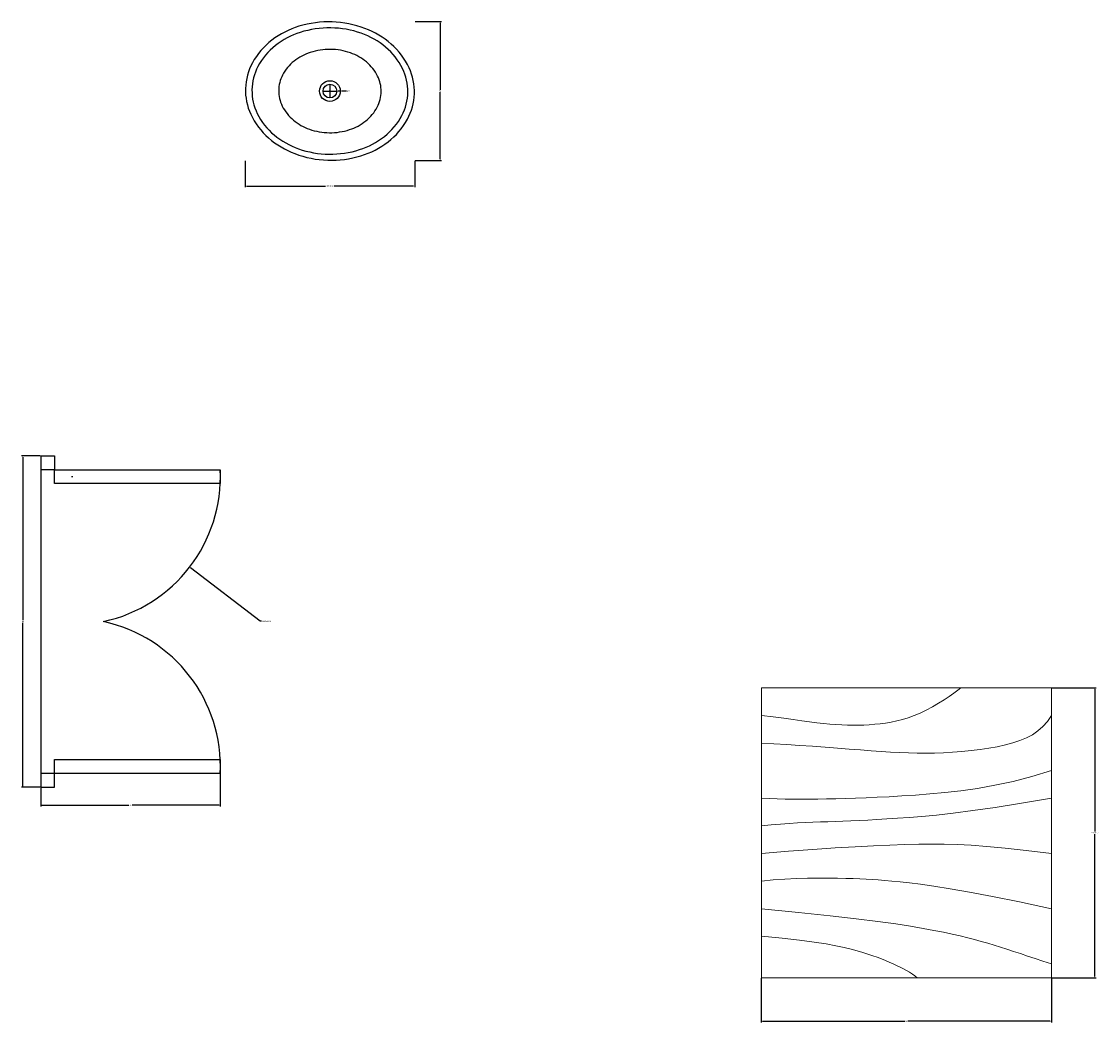
# Model space of a CAD drawing. Units: inches. Extents: x 821 to 2399, y 74 to 823.
# Tile 9 of 13: x 1922 to 2078, y 193 to 338. Entities that reach past the tile are written whole.
import ezdxf

# ---------------------------------------------------------------- set-up
doc = ezdxf.new("R2010")
doc.units = ezdxf.units.IN
doc.header["$MEASUREMENT"] = 0
doc.layers.get('0').update_dxf_attribs({"lineweight": 53})
for name, color, linetype, lineweight in [('A-ANNO-DIMS', 2, 'Continuous', 18), ('A-DOOR', 4, 'Continuous', 25), ('A-FLOR-FIXT', 8, 'Continuous', 25), ('A-FURN', 8, 'Continuous', 18)]:
    doc.layers.add(name, color=color, linetype=linetype, lineweight=lineweight)
doc.styles.get("Standard").update_dxf_attribs({"font": 'arial.ttf'})
doc.dimstyles.get("Standard").update_dxf_attribs({"dimtxt": 0.18, "dimasz": 0.18, "dimexe": 0.18, "dimexo": 0.0625, "dimgap": 0.09, "dimtad": 0, "dimtih": 1, "dimtoh": 1, "dimdec": 4, "dimzin": 0, "dimdsep": 46, "dimtxsty": 'Standard', "dimcen": 0.09, "dimadec": 0, "dimazin": 0, "dimtfac": 1, "dimtdec": 4, "dimtofl": 0, "dimtmove": 0, "dimatfit": 3, "dimfxl": 1, "dimtolj": 1, "dimtzin": 0, "dimarcsym": 0})

# ---------------------------------------------------------------- blocks, each defined once
blk = doc.blocks.new('Table - Square Woodgrain 42 x 42 in.')
blk.add_line((0, -42), (42, -42))
for points in [[(0, -4), (1.704, -4.2172), (3.2358, -4.4188), (4.615, -4.604), (5.8615, -4.7721), (6.9951, -4.9224), (8.0357, -5.0541), (9.0031, -5.1667), (9.9171, -5.2594), (10.7951, -5.3316), (11.6445, -5.3836), (12.4702, -5.4157), (13.277, -5.4283), (14.0698, -5.4217), (14.8535, -5.3964), (15.6331, -5.3526), (16.4133, -5.2908), (17.1986, -5.2103), (17.9913, -5.1062), (18.793, -4.9727), (19.6056, -4.8038), (20.4307, -4.5937), (21.2701, -4.3365), (22.1256, -4.0262), (22.9989, -3.6571), (23.888, -3.2272), (24.7756, -2.7516), (25.6408, -2.2491), (26.4624, -1.7387), (27.2195, -1.2395), (27.891, -0.7703), (28.456, -0.3501), (28.8934, 0.002)], [(0, -42), (0, 0), (42, 0), (42, -42)], [(0, -8), (1.8203, -8.1001), (3.6741, -8.2149), (5.5411, -8.3408), (7.4011, -8.4741), (9.2339, -8.6112), (11.0193, -8.7484), (12.7371, -8.8821), (14.3671, -9.0086), (15.8954, -9.1246), (17.3337, -9.2278), (18.6997, -9.3159), (20.0116, -9.387), (21.2871, -9.4389), (22.5442, -9.4696), (23.8008, -9.477), (25.0749, -9.459), (26.3791, -9.4137), (27.7049, -9.3403), (29.0383, -9.2382), (30.3655, -9.1068), (31.6728, -8.9455), (32.9461, -8.7535), (34.1717, -8.5304), (35.3358, -8.2756), (36.4268, -7.9863), (37.443, -7.6521), (38.3849, -7.2603), (39.253, -6.7986), (40.048, -6.2542), (40.7705, -5.6147), (41.421, -4.8674), (42, -4)], [(42, -12), (39.1784, -12.8621), (36.4519, -13.5654), (33.8246, -14.1294), (31.3004, -14.5731), (28.8832, -14.9161), (26.577, -15.1775), (24.3858, -15.3768), (22.3136, -15.5332), (20.3622, -15.6632), (18.5254, -15.7718), (16.7947, -15.8612), (15.1618, -15.9338), (13.6183, -15.9916), (12.1558, -16.0369), (10.7659, -16.0718), (9.4403, -16.0987), (8.1703, -16.1191), (6.9461, -16.1325), (5.7577, -16.1377), (4.595, -16.1335), (3.4479, -16.1188), (2.3064, -16.0924), (1.1604, -16.0532), (0, -16)], [(42, -16), (37.6529, -16.7365), (33.8802, -17.329), (30.6179, -17.7961), (27.8015, -18.1561), (25.3668, -18.4275), (23.2497, -18.6288), (21.3859, -18.7785), (19.7111, -18.8949), (18.1693, -18.9939), (16.7375, -19.0795), (15.401, -19.1534), (14.1449, -19.217), (12.9544, -19.2717), (11.8148, -19.3191), (10.7113, -19.3606), (9.6291, -19.3976), (8.5534, -19.4323), (7.47, -19.4689), (6.3643, -19.5122), (5.222, -19.5672), (4.0288, -19.6386), (2.7703, -19.7313), (1.4321, -19.8501), (0, -20)], [(0, -24), (3.9243, -23.6805), (7.4766, -23.4138), (10.6891, -23.1954), (13.5943, -23.0205), (16.2247, -22.8847), (18.6125, -22.7832), (20.7903, -22.7116), (22.7903, -22.6651), (24.6563, -22.642), (26.4764, -22.6507), (28.35, -22.7024), (30.3766, -22.8084), (32.6555, -22.98), (35.2861, -23.2283), (38.3678, -23.5645), (42, -24)], [(42, -32), (37.392, -31.017), (33.4585, -30.2231), (30.1291, -29.5949), (27.3334, -29.109), (25.0009, -28.742), (23.0612, -28.4707), (21.4439, -28.2716), (20.0786, -28.1215), (18.8998, -28.0002), (17.8609, -27.9014), (16.9206, -27.8219), (16.0371, -27.7588), (15.1691, -27.709), (14.2748, -27.6693), (13.3128, -27.6368), (12.2415, -27.6083), (11.0295, -27.5824), (9.6867, -27.5643), (8.233, -27.5608), (6.6884, -27.5787), (5.0728, -27.6248), (3.4062, -27.7058), (1.7086, -27.8286), (0, -28)], [(0, -32), (5.4026, -32.5358), (9.9494, -33.019), (13.7424, -33.4553), (16.8834, -33.8505), (19.4743, -34.2106), (21.6171, -34.5413), (23.4136, -34.8486), (24.9657, -35.1382), (26.3614, -35.4156), (27.6332, -35.6841), (28.7995, -35.9467), (29.8788, -36.2064), (30.8897, -36.4661), (31.8507, -36.7288), (32.7802, -36.9973), (33.6968, -37.2747), (34.6175, -37.5635), (35.5531, -37.8651), (36.5128, -38.1805), (37.506, -38.5108), (38.5421, -38.8568), (39.6302, -39.2197), (40.7797, -39.6004), (42, -40)], [(0, -36), (3.0098, -36.2857), (5.5354, -36.5643), (7.6368, -36.8359), (9.374, -37.1009), (10.807, -37.3597), (11.9957, -37.6126), (13.0002, -37.8599), (13.8804, -38.102), (14.6874, -38.3393), (15.4365, -38.5729), (16.1338, -38.8041), (16.7858, -39.0341), (17.3987, -39.264), (17.9787, -39.4952), (18.5322, -39.7288), (19.0655, -39.9662), (19.5832, -40.2081), (20.0842, -40.4544), (20.5657, -40.7046), (21.0249, -40.9581), (21.459, -41.2144), (21.8653, -41.4731), (22.2409, -41.7335), (22.5831, -41.9951)]]:
    blk.add_lwpolyline(points)
blk = doc.blocks.new('Sink - Oval top')
for p, q in [((-1, 0), (1, 0)), ((0, 1), (0, -1))]:
    blk.add_line(p, q)
for points in [[(-12.23, 0.39, 0.117634), (-11.46, -3.36, 0.104469), (-8.88, -6.8, 0.090016), (-5.08, -9.07, 0.08192), (-0.32, -10.02, 0.08192), (4.49, -9.38, 0.090016), (8.42, -7.36, 0.104469), (11.22, -4.09, 0.117634), (12.23, -0.39, 0.117634), (11.46, 3.36, 0.104469), (8.88, 6.8, 0.090016), (5.08, 9.07, 0.08192), (0.32, 10.02, 0.08192), (-4.49, 9.38, 0.090016), (-8.42, 7.36, 0.104469), (-11.22, 4.09, 0.117634)], [(-11.29, 0.16, 0.118622), (-10.52, -3.25, 0.104678), (-8.07, -6.36, 0.089562), (-4.54, -8.37, 0.081185), (-0.13, -9.15, 0.081185), (4.3, -8.49, 0.089562), (7.89, -6.58, 0.104678), (10.42, -3.55, 0.118622), (11.29, -0.16, 0.118622), (10.52, 3.25, 0.104678), (8.07, 6.36, 0.089562), (4.54, 8.37, 0.081185), (0.13, 9.15, 0.081185), (-4.3, 8.49, 0.089562), (-7.89, 6.58, 0.104678), (-10.42, 3.55, 0.118622)], [(-7.42, 0.08, 0.118283), (-6.91, -2.17, 0.104607), (-5.29, -4.21, 0.089718), (-2.97, -5.53, 0.081436), (-0.07, -6.04, 0.081436), (2.84, -5.59, 0.089718), (5.2, -4.33, 0.104607), (6.86, -2.32, 0.118283), (7.42, -0.08, 0.118283), (6.91, 2.17, 0.104607), (5.29, 4.21, 0.089718), (2.97, 5.53, 0.081436), (0.07, 6.04, 0.081436), (-2.84, 5.59, 0.089718), (-5.2, 4.33, 0.104607), (-6.86, 2.32, 0.118283)]]:
    blk.add_lwpolyline(points, format="xyb", close=True)
for radius in [1.5, 1]:
    blk.add_circle((0, 0), radius)
blk = doc.blocks.new('*D70')
at = {"layer": 'A-ANNO-DIMS', "color": 0, "lineweight": -2, "transparency": 16777216}
for p, q in [((2071.03, 241.41), (2077.44, 241.41)), ((2077.26, 241.23), (2077.26, 220.59)), ((2077.26, 199.59), (2077.26, 220.23)), ((2071.03, 199.41), (2077.44, 199.41))]:
    blk.add_line(p, q, dxfattribs=at)
at = {"layer": 'A-ANNO-DIMS', "color": 0, "lineweight": 50, "transparency": 16777216}
for points in [[(2077.23, 241.23), (2077.29, 241.23), (2077.26, 241.41)], [(2077.23, 199.59), (2077.29, 199.59), (2077.26, 199.41)]]:
    blk.add_solid(points, dxfattribs=at)
at = {"layer": 'Defpoints', "color": 0, "lineweight": 50, "transparency": 16777216}
for p in [(2070.96, 241.41), (2077.26, 241.41), (2070.96, 199.41)]:
    blk.add_point(p, dxfattribs=at)
at = {"layer": 'A-ANNO-DIMS', "color": 0, "transparency": 16777216, "insert": (2077.26, 220.41), "char_height": 0.18, "attachment_point": 5}
blk.add_mtext('\\A1;TABLE 42', dxfattribs=at)
blk = doc.blocks.new('*D71')
at = {"layer": 'A-ANNO-DIMS', "color": 0, "lineweight": -2, "transparency": 16777216}
for p, q in [((2028.96, 199.35), (2028.96, 192.93)), ((2070.96, 199.35), (2070.96, 192.93)), ((2029.14, 193.11), (2049.74, 193.11)), ((2070.78, 193.11), (2050.19, 193.11))]:
    blk.add_line(p, q, dxfattribs=at)
at = {"layer": 'A-ANNO-DIMS', "color": 0, "lineweight": 50, "transparency": 16777216}
for points in [[(2029.14, 193.14), (2029.14, 193.08), (2028.96, 193.11)], [(2070.78, 193.14), (2070.78, 193.08), (2070.96, 193.11)]]:
    blk.add_solid(points, dxfattribs=at)
at = {"layer": 'Defpoints', "color": 0, "lineweight": 50, "transparency": 16777216}
for p in [(2028.96, 199.41), (2070.96, 199.41), (2070.96, 193.11)]:
    blk.add_point(p, dxfattribs=at)
at = {"layer": 'A-ANNO-DIMS', "color": 0, "transparency": 16777216, "insert": (2049.96, 193.11), "char_height": 0.18, "attachment_point": 5}
blk.add_mtext('\\A1;42', dxfattribs=at)
blk = doc.blocks.new('*D72')
at = {"layer": 'A-ANNO-DIMS', "color": 0, "lineweight": -2, "transparency": 16777216}
for p, q in [((1954.21, 317.73), (1954.21, 313.92)), ((1978.76, 317.73), (1978.76, 313.92)), ((1954.39, 314.1), (1965.85, 314.1)), ((1978.58, 314.1), (1967.11, 314.1))]:
    blk.add_line(p, q, dxfattribs=at)
at = {"layer": 'A-ANNO-DIMS', "color": 0, "lineweight": 50, "transparency": 16777216}
for points in [[(1954.39, 314.13), (1954.39, 314.07), (1954.21, 314.1)], [(1978.58, 314.13), (1978.58, 314.07), (1978.76, 314.1)]]:
    blk.add_solid(points, dxfattribs=at)
at = {"layer": 'Defpoints', "color": 0, "lineweight": 50, "transparency": 16777216}
for p in [(1954.21, 317.79), (1978.76, 317.79), (1978.76, 314.1)]:
    blk.add_point(p, dxfattribs=at)
at = {"layer": 'A-ANNO-DIMS', "color": 0, "transparency": 16777216, "insert": (1966.48, 314.1), "char_height": 0.18, "attachment_point": 5}
blk.add_mtext('\\A1;BASIN 25', dxfattribs=at)
blk = doc.blocks.new('*D73')
at = {"layer": 'A-ANNO-DIMS', "color": 0, "lineweight": -2, "transparency": 16777216}
for p, q in [((1978.82, 337.92), (1982.62, 337.92)), ((1982.44, 337.74), (1982.44, 328.04)), ((1982.44, 317.97), (1982.44, 327.67)), ((1978.82, 317.79), (1982.62, 317.79))]:
    blk.add_line(p, q, dxfattribs=at)
at = {"layer": 'A-ANNO-DIMS', "color": 0, "lineweight": 50, "transparency": 16777216}
for points in [[(1982.41, 337.74), (1982.47, 337.74), (1982.44, 337.92)], [(1982.41, 317.97), (1982.47, 317.97), (1982.44, 317.79)]]:
    blk.add_solid(points, dxfattribs=at)
at = {"layer": 'Defpoints', "color": 0, "lineweight": 50, "transparency": 16777216}
for p in [(1978.76, 337.92), (1982.44, 337.92), (1978.76, 317.79)]:
    blk.add_point(p, dxfattribs=at)
at = {"layer": 'A-ANNO-DIMS', "color": 0, "transparency": 16777216, "insert": (1982.44, 327.86), "char_height": 0.18, "attachment_point": 5}
blk.add_mtext('\\A1;20', dxfattribs=at)
blk = doc.blocks.new('*D128')
at = {"layer": 'A-ANNO-DIMS', "color": 0, "lineweight": -2, "transparency": 16777216}
for p, q in [((1924.54, 275), (1921.82, 275)), ((1922, 274.82), (1922, 251.19)), ((1922, 227.18), (1922, 250.82)), ((1924.54, 227), (1921.82, 227))]:
    blk.add_line(p, q, dxfattribs=at)
at = {"layer": 'A-ANNO-DIMS', "color": 0, "lineweight": 50, "transparency": 16777216}
for points in [[(1921.97, 274.82), (1922.03, 274.82), (1922, 275)], [(1921.97, 227.18), (1922.03, 227.18), (1922, 227)]]:
    blk.add_solid(points, dxfattribs=at)
at = {"layer": 'Defpoints', "color": 0, "lineweight": 50, "transparency": 16777216}
for p in [(1922, 275), (1924.6, 275), (1924.6, 227)]:
    blk.add_point(p, dxfattribs=at)
at = {"layer": 'A-ANNO-DIMS', "color": 0, "transparency": 16777216, "insert": (1922, 251), "char_height": 0.18, "attachment_point": 5}
blk.add_mtext('\\A1;48', dxfattribs=at)
blk = doc.blocks.new('*D129')
at = {"layer": 'A-ANNO-DIMS', "color": 0, "lineweight": -2, "transparency": 16777216}
for p, q in [((1950.6, 228.94), (1950.6, 224.22)), ((1924.6, 226.94), (1924.6, 224.22)), ((1924.78, 224.4), (1937.38, 224.4)), ((1950.42, 224.4), (1937.82, 224.4))]:
    blk.add_line(p, q, dxfattribs=at)
at = {"layer": 'A-ANNO-DIMS', "color": 0, "lineweight": 50, "transparency": 16777216}
for points in [[(1924.78, 224.43), (1924.78, 224.37), (1924.6, 224.4)], [(1950.42, 224.43), (1950.42, 224.37), (1950.6, 224.4)]]:
    blk.add_solid(points, dxfattribs=at)
at = {"layer": 'Defpoints', "color": 0, "lineweight": 50, "transparency": 16777216}
for p in [(1950.6, 229), (1924.6, 227), (1950.6, 224.4)]:
    blk.add_point(p, dxfattribs=at)
at = {"layer": 'A-ANNO-DIMS', "color": 0, "transparency": 16777216, "insert": (1937.6, 224.4), "char_height": 0.18, "attachment_point": 5}
blk.add_mtext('\\A1;26', dxfattribs=at)
blk = doc.blocks.new('*D150')
at = {"layer": 'A-ANNO-DIMS', "color": 0, "lineweight": -2, "transparency": 16777216}
for p, q in [((1929.05, 272), (1929.23, 272)), ((1929.14, 271.91), (1929.14, 272.09)), ((1956.39, 251.05), (1946.31, 258.8)), ((1956.57, 251.05), (1956.39, 251.05))]:
    blk.add_line(p, q, dxfattribs=at)
at = {"layer": 'A-ANNO-DIMS', "color": 0, "lineweight": 50, "transparency": 16777216}
blk.add_solid([(1946.33, 258.82), (1946.29, 258.77), (1946.17, 258.91)], dxfattribs=at)
at = {"layer": 'Defpoints', "color": 0, "lineweight": 50, "transparency": 16777216}
for p in [(1929.14, 272), (1946.17, 258.91)]:
    blk.add_point(p, dxfattribs=at)
at = {"layer": 'A-ANNO-DIMS', "color": 0, "transparency": 16777216, "insert": (1957.31, 251.05), "char_height": 0.18, "attachment_point": 5}
blk.add_mtext('\\A1;2X R21.485', dxfattribs=at)
blk = doc.blocks.new('*D154')
at = {"layer": 'A-ANNO-DIMS', "color": 0, "lineweight": -2, "transparency": 16777216}
for p, q in [((1966.39, 327.86), (1966.57, 327.86)), ((1966.48, 327.77), (1966.48, 327.95)), ((1968.88, 327.86), (1968.16, 327.86))]:
    blk.add_line(p, q, dxfattribs=at)
at = {"layer": 'A-ANNO-DIMS', "color": 0, "lineweight": 50, "transparency": 16777216}
blk.add_solid([(1968.16, 327.89), (1968.16, 327.83), (1967.98, 327.86)], dxfattribs=at)
at = {"layer": 'Defpoints', "color": 0, "lineweight": 50, "transparency": 16777216}
for p in [(1964.98, 327.86), (1967.98, 327.86)]:
    blk.add_point(p, dxfattribs=at)
at = {"layer": 'A-ANNO-DIMS', "color": 0, "transparency": 16777216, "insert": (1969.13, 327.86), "char_height": 0.18, "attachment_point": 5}
blk.add_mtext('\\A1;∅3', dxfattribs=at)
blk = doc.blocks.new('*D155')
at = {"layer": 'A-ANNO-DIMS', "color": 0, "lineweight": -2, "transparency": 16777216}
for p, q in [((1966.39, 327.86), (1966.57, 327.86)), ((1966.48, 327.77), (1966.48, 327.95)), ((1968.08, 327.86), (1967.66, 327.86))]:
    blk.add_line(p, q, dxfattribs=at)
at = {"layer": 'A-ANNO-DIMS', "color": 0, "lineweight": 50, "transparency": 16777216}
blk.add_solid([(1967.66, 327.89), (1967.66, 327.83), (1967.48, 327.86)], dxfattribs=at)
at = {"layer": 'Defpoints', "color": 0, "lineweight": 50, "transparency": 16777216}
for p in [(1965.48, 327.86), (1967.48, 327.86)]:
    blk.add_point(p, dxfattribs=at)
at = {"layer": 'A-ANNO-DIMS', "color": 0, "transparency": 16777216, "insert": (1968.33, 327.86), "char_height": 0.18, "attachment_point": 5}
blk.add_mtext('\\A1;∅2', dxfattribs=at)

msp = doc.modelspace()

# ---------------------------------------------------------------- linework, layer by layer
at = {"layer": 'A-DOOR'}
for p, q in [((1924.6021, 275.0047), (1924.6021, 227.0047)), ((1924.6021, 275.0047), (1926.6021, 275.0047)), ((1926.6021, 275.0047), (1926.6021, 273.0047)), ((1926.6021, 273.0047), (1924.6021, 273.0047)), ((1926.6021, 273.0047), (1950.6021, 273.0047)), ((1926.6021, 271.0047), (1926.6021, 273.0047)), ((1950.6021, 273.0047), (1950.6021, 271.0047)), ((1950.6021, 271.0047), (1926.6021, 271.0047)), ((1926.6021, 229.0047), (1926.6021, 231.0047)), ((1926.6021, 231.0047), (1950.6021, 231.0047)), ((1950.6021, 231.0047), (1950.6021, 229.0047)), ((1926.6021, 229.0047), (1924.6021, 229.0047)), ((1926.6021, 227.0047), (1926.6021, 229.0047)), ((1950.6021, 229.0047), (1926.6021, 229.0047)), ((1924.6021, 227.0047), (1926.6021, 227.0047))]:
    msp.add_line(p, q, dxfattribs=at)
for centre, start, end in [((1929.1406, 272.0047), 282.19505, 2.667766), ((1929.1406, 230.0047), 357.332234, 77.80495)]:
    msp.add_arc(centre, 21.4848, start, end, dxfattribs=at)

# ---------------------------------------------------------------- block references
at = {"layer": 'A-FLOR-FIXT'}
msp.add_blockref('Sink - Oval top', (1966.4817, 327.8559), dxfattribs=at)
at = {"layer": 'A-FURN'}
msp.add_blockref('Table - Square Woodgrain 42 x 42 in.', (2028.9641, 241.4126), dxfattribs=at)

# ---------------------------------------------------------------- dimensions: what is measured, and where the dimension line sits
at = {"layer": 'A-ANNO-DIMS'}
for base, p1, p2, picture, middle in [((1982.4398, 337.9242), (1978.7571, 317.7876), (1978.7571, 337.9242), '*D73', (1982.4398, 327.8559)), ((1922.0021, 275.0047), (1924.6021, 227.0047), (1924.6021, 275.0047), '*D128', (1922.0021, 251.0047))]:
    dim = msp.add_linear_dim(base=base, p1=p1, p2=p2, angle=90, dimstyle='Standard', override={"dimdec": 0, "dimlfac": 1, "dimrnd": 0, "dimzin": 0, "dimdsep": 46, "dimlunit": 2}, dxfattribs=at)
    dim.commit()
    dim.dimension.update_dxf_attribs({"geometry": picture, "text_midpoint": middle})
for p1, p2, picture, middle in [((1964.9817, 327.8558), (1967.9817, 327.856), '*D154', (1968.8817, 327.856)), ((1965.4817, 327.8558), (1967.4817, 327.856), '*D155', (1968.0817, 327.856))]:
    dim = msp.add_diameter_dim_2p(p1=p1, p2=p2, dimstyle='Standard', override={"dimdec": 0, "dimlfac": 1, "dimrnd": 0, "dimzin": 0, "dimdsep": 46, "dimlunit": 2}, dxfattribs=at)
    dim.commit()
    dim.dimension.update_dxf_attribs({"geometry": picture, "text_midpoint": middle, "dimtype": 163})
dim = msp.add_linear_dim(base=(1978.7571, 314.105), p1=(1954.2062, 317.7876), p2=(1978.7571, 317.7876), text='BASIN <>', dimstyle='Standard', override={"dimdec": 0, "dimlfac": 1, "dimrnd": 0, "dimzin": 0, "dimdsep": 46, "dimlunit": 2}, dxfattribs=at)
dim.commit()
dim.dimension.update_dxf_attribs({"geometry": '*D72', "text_midpoint": (1966.4817, 314.105)})
dim = msp.add_radius_dim(center=(1929.1406, 272.0047), mpoint=(1946.1699, 258.9051), text='2X <>', dimstyle='Standard', override={"dimdec": 3, "dimlfac": 1, "dimrnd": 0, "dimzin": 0, "dimdsep": 46, "dimlunit": 2}, dxfattribs=at)
dim.commit()
dim.dimension.update_dxf_attribs({"geometry": '*D150', "text_midpoint": (1957.3128, 251.0453), "dimtype": 164})
dim = msp.add_linear_dim(base=(2077.2644, 241.4146), p1=(2070.9641, 199.4126), p2=(2070.9641, 241.4146), angle=90, text='TABLE <>', dimstyle='Standard', override={"dimdec": 0, "dimlfac": 1, "dimrnd": 0, "dimzin": 0, "dimdsep": 46, "dimlunit": 2}, dxfattribs=at)
dim.commit()
dim.dimension.update_dxf_attribs({"geometry": '*D70', "text_midpoint": (2077.2644, 220.4136)})
for base, p1, p2, picture, middle in [((1950.6021, 224.4047), (1924.6021, 227.0047), (1950.6021, 229.0047), '*D129', (1937.6021, 224.4047)), ((2070.9641, 193.1123), (2028.9641, 199.4126), (2070.9641, 199.4126), '*D71', (2049.9641, 193.1123))]:
    dim = msp.add_linear_dim(base=base, p1=p1, p2=p2, dimstyle='Standard', override={"dimdec": 0, "dimlfac": 1, "dimrnd": 0, "dimzin": 0, "dimdsep": 46, "dimlunit": 2}, dxfattribs=at)
    dim.commit()
    dim.dimension.update_dxf_attribs({"geometry": picture, "text_midpoint": middle})

doc.saveas('drawing.dxf')
